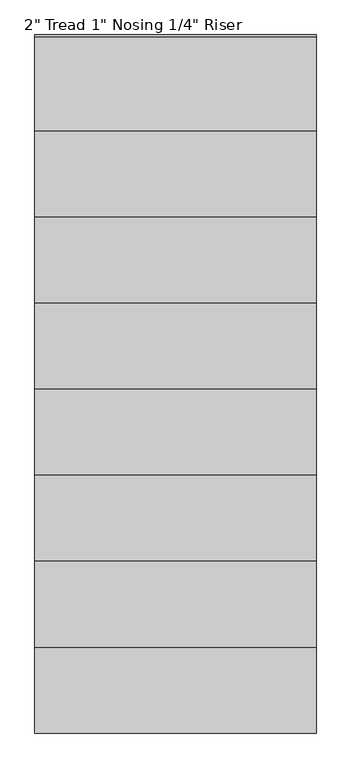
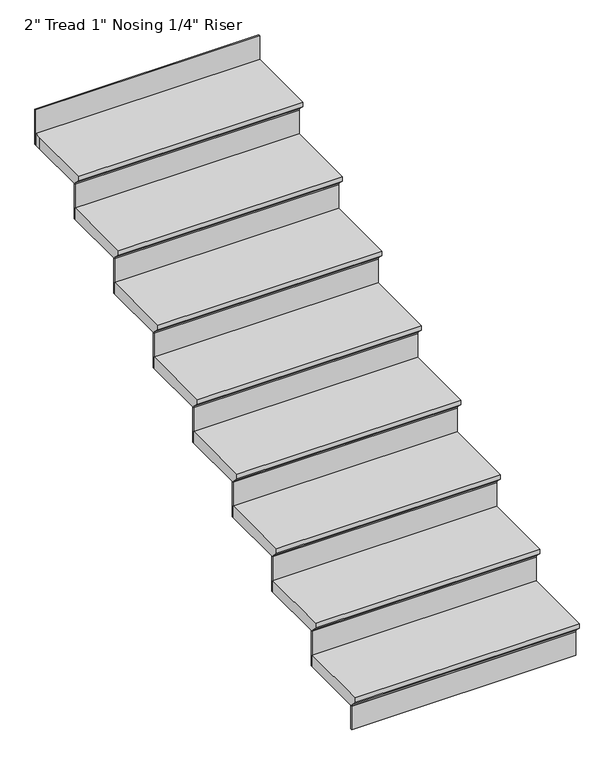
"""IFC4 building model written with IfcOpenShell, lengths in millimetres: stair flight geometry."""

from ifc_helpers import new_model, si_unit, origin, place, context, project, spatial, faceted_brep, source, transform, mapped, element, save


def stair_flight_7b1ec15d(model_context):
    return source(origin(), model_context, "Body", "Brep", [
        faceted_brep([(1196.7463194, 2224.4726898, 133.35), (1196.7463194, 2224.4726898, 152.4), (282.3463194, 2224.4726898, 152.4), (282.3463194, 2224.4726898, 133.35), (1196.7463194, 2249.8726898, 107.95), (282.3463194, 2249.8726898, 107.95), (1196.7463194, 2529.2726898, 152.4), (282.3463194, 2529.2726898, 152.4), (282.3463194, 2249.8726898, 101.6), (282.3463194, 2529.2726898, 101.6), (1196.7463194, 2529.2726898, 101.6), (1196.7463194, 2249.8726898, 101.6)], [[[0, 1, 2, 3]], [[4, 0, 3, 5]], [[2, 1, 6, 7]], [[8, 9, 10, 11]], [[2, 7, 9, 8, 5, 3]], [[8, 11, 4, 5]], [[6, 1, 0, 4, 11, 10]], [[7, 6, 10, 9]]]),
        faceted_brep([(1196.7463194, 2249.8726898, 101.6), (1196.7463194, 2249.8726898, 0.0), (1196.7463194, 2256.2226898, 0.0), (1196.7463194, 2256.2226898, 101.6), (282.3463194, 2249.8726898, 101.6), (282.3463194, 2256.2226898, 101.6), (282.3463194, 2256.2226898, 0.0), (282.3463194, 2249.8726898, 0.0)], [[[0, 1, 2, 3]], [[4, 5, 6, 7]], [[1, 0, 4, 7]], [[2, 1, 7, 6]], [[3, 2, 6, 5]], [[0, 3, 5, 4]]]),
        faceted_brep([(1196.7463194, 2529.2726898, 254.0), (1196.7463194, 2529.2726898, 101.6), (1196.7463194, 2535.6226898, 101.6), (1196.7463194, 2535.6226898, 254.0), (282.3463194, 2529.2726898, 254.0), (282.3463194, 2535.6226898, 254.0), (282.3463194, 2535.6226898, 101.6), (282.3463194, 2529.2726898, 101.6)], [[[0, 1, 2, 3]], [[4, 5, 6, 7]], [[1, 0, 4, 7]], [[2, 1, 7, 6]], [[3, 2, 6, 5]], [[0, 3, 5, 4]]]),
        faceted_brep([(282.3463194, 2503.8726898, 304.8), (1196.7463194, 2503.8726898, 304.8), (1196.7463194, 2808.6726898, 304.8), (282.3463194, 2808.6726898, 304.8), (282.3463194, 2529.2726898, 254.0), (282.3463194, 2808.6726898, 254.0), (1196.7463194, 2808.6726898, 254.0), (1196.7463194, 2529.2726898, 254.0), (282.3463194, 2529.2726898, 260.35), (282.3463194, 2503.8726898, 285.75), (1196.7463194, 2529.2726898, 260.35), (1196.7463194, 2503.8726898, 285.75)], [[[0, 1, 2, 3]], [[4, 5, 6, 7]], [[0, 3, 5, 4, 8, 9]], [[4, 7, 10, 8]], [[2, 1, 11, 10, 7, 6]], [[3, 2, 6, 5]], [[11, 1, 0, 9]], [[10, 11, 9, 8]]]),
        faceted_brep([(1196.7463194, 2808.6726898, 406.4), (1196.7463194, 2808.6726898, 254.0), (1196.7463194, 2815.0226898, 254.0), (1196.7463194, 2815.0226898, 406.4), (282.3463194, 2808.6726898, 406.4), (282.3463194, 2815.0226898, 406.4), (282.3463194, 2815.0226898, 254.0), (282.3463194, 2808.6726898, 254.0)], [[[0, 1, 2, 3]], [[4, 5, 6, 7]], [[1, 0, 4, 7]], [[2, 1, 7, 6]], [[3, 2, 6, 5]], [[0, 3, 5, 4]]]),
        faceted_brep([(282.3463194, 2783.2726898, 457.2), (1196.7463194, 2783.2726898, 457.2), (1196.7463194, 3088.0726898, 457.2), (282.3463194, 3088.0726898, 457.2), (282.3463194, 2808.6726898, 406.4), (282.3463194, 3088.0726898, 406.4), (1196.7463194, 3088.0726898, 406.4), (1196.7463194, 2808.6726898, 406.4), (282.3463194, 2808.6726898, 412.75), (282.3463194, 2783.2726898, 438.15), (1196.7463194, 2808.6726898, 412.75), (1196.7463194, 2783.2726898, 438.15)], [[[0, 1, 2, 3]], [[4, 5, 6, 7]], [[0, 3, 5, 4, 8, 9]], [[4, 7, 10, 8]], [[2, 1, 11, 10, 7, 6]], [[3, 2, 6, 5]], [[11, 1, 0, 9]], [[10, 11, 9, 8]]]),
        faceted_brep([(1196.7463194, 3088.0726898, 558.8), (1196.7463194, 3088.0726898, 406.4), (1196.7463194, 3094.4226898, 406.4), (1196.7463194, 3094.4226898, 558.8), (282.3463194, 3088.0726898, 558.8), (282.3463194, 3094.4226898, 558.8), (282.3463194, 3094.4226898, 406.4), (282.3463194, 3088.0726898, 406.4)], [[[0, 1, 2, 3]], [[4, 5, 6, 7]], [[1, 0, 4, 7]], [[2, 1, 7, 6]], [[3, 2, 6, 5]], [[0, 3, 5, 4]]]),
        faceted_brep([(282.3463194, 3062.6726898, 609.6), (1196.7463194, 3062.6726898, 609.6), (1196.7463194, 3367.4726898, 609.6), (282.3463194, 3367.4726898, 609.6), (282.3463194, 3088.0726898, 558.8), (282.3463194, 3367.4726898, 558.8), (1196.7463194, 3367.4726898, 558.8), (1196.7463194, 3088.0726898, 558.8), (282.3463194, 3088.0726898, 565.15), (282.3463194, 3062.6726898, 590.55), (1196.7463194, 3088.0726898, 565.15), (1196.7463194, 3062.6726898, 590.55)], [[[0, 1, 2, 3]], [[4, 5, 6, 7]], [[0, 3, 5, 4, 8, 9]], [[4, 7, 10, 8]], [[2, 1, 11, 10, 7, 6]], [[3, 2, 6, 5]], [[11, 1, 0, 9]], [[10, 11, 9, 8]]]),
        faceted_brep([(1196.7463194, 3367.4726898, 711.2), (1196.7463194, 3367.4726898, 558.8), (1196.7463194, 3373.8226898, 558.8), (1196.7463194, 3373.8226898, 711.2), (282.3463194, 3367.4726898, 711.2), (282.3463194, 3373.8226898, 711.2), (282.3463194, 3373.8226898, 558.8), (282.3463194, 3367.4726898, 558.8)], [[[0, 1, 2, 3]], [[4, 5, 6, 7]], [[1, 0, 4, 7]], [[2, 1, 7, 6]], [[3, 2, 6, 5]], [[0, 3, 5, 4]]]),
        faceted_brep([(282.3463194, 3342.0726898, 762.0), (1196.7463194, 3342.0726898, 762.0), (1196.7463194, 3646.8726898, 762.0), (282.3463194, 3646.8726898, 762.0), (282.3463194, 3367.4726898, 711.2), (282.3463194, 3646.8726898, 711.2), (1196.7463194, 3646.8726898, 711.2), (1196.7463194, 3367.4726898, 711.2), (282.3463194, 3367.4726898, 717.55), (282.3463194, 3342.0726898, 742.95), (1196.7463194, 3367.4726898, 717.55), (1196.7463194, 3342.0726898, 742.95)], [[[0, 1, 2, 3]], [[4, 5, 6, 7]], [[0, 3, 5, 4, 8, 9]], [[4, 7, 10, 8]], [[2, 1, 11, 10, 7, 6]], [[3, 2, 6, 5]], [[11, 1, 0, 9]], [[10, 11, 9, 8]]]),
        faceted_brep([(1196.7463194, 3646.8726898, 863.6), (1196.7463194, 3646.8726898, 711.2), (1196.7463194, 3653.2226898, 711.2), (1196.7463194, 3653.2226898, 863.6), (282.3463194, 3646.8726898, 863.6), (282.3463194, 3653.2226898, 863.6), (282.3463194, 3653.2226898, 711.2), (282.3463194, 3646.8726898, 711.2)], [[[0, 1, 2, 3]], [[4, 5, 6, 7]], [[1, 0, 4, 7]], [[2, 1, 7, 6]], [[3, 2, 6, 5]], [[0, 3, 5, 4]]]),
        faceted_brep([(282.3463194, 3621.4726898, 914.4), (1196.7463194, 3621.4726898, 914.4), (1196.7463194, 3926.2726898, 914.4), (282.3463194, 3926.2726898, 914.4), (282.3463194, 3646.8726898, 863.6), (282.3463194, 3926.2726898, 863.6), (1196.7463194, 3926.2726898, 863.6), (1196.7463194, 3646.8726898, 863.6), (282.3463194, 3646.8726898, 869.95), (282.3463194, 3621.4726898, 895.35), (1196.7463194, 3646.8726898, 869.95), (1196.7463194, 3621.4726898, 895.35)], [[[0, 1, 2, 3]], [[4, 5, 6, 7]], [[0, 3, 5, 4, 8, 9]], [[4, 7, 10, 8]], [[2, 1, 11, 10, 7, 6]], [[3, 2, 6, 5]], [[11, 1, 0, 9]], [[10, 11, 9, 8]]]),
        faceted_brep([(1196.7463194, 3926.2726898, 1016.0), (1196.7463194, 3926.2726898, 863.6), (1196.7463194, 3932.6226898, 863.6), (1196.7463194, 3932.6226898, 1016.0), (282.3463194, 3926.2726898, 1016.0), (282.3463194, 3932.6226898, 1016.0), (282.3463194, 3932.6226898, 863.6), (282.3463194, 3926.2726898, 863.6)], [[[0, 1, 2, 3]], [[4, 5, 6, 7]], [[1, 0, 4, 7]], [[2, 1, 7, 6]], [[3, 2, 6, 5]], [[0, 3, 5, 4]]]),
        faceted_brep([(282.3463194, 3900.8726898, 1066.8), (1196.7463194, 3900.8726898, 1066.8), (1196.7463194, 4205.6726898, 1066.8), (282.3463194, 4205.6726898, 1066.8), (282.3463194, 3926.2726898, 1016.0), (282.3463194, 4205.6726898, 1016.0), (1196.7463194, 4205.6726898, 1016.0), (1196.7463194, 3926.2726898, 1016.0), (282.3463194, 3926.2726898, 1022.35), (282.3463194, 3900.8726898, 1047.75), (1196.7463194, 3926.2726898, 1022.35), (1196.7463194, 3900.8726898, 1047.75)], [[[0, 1, 2, 3]], [[4, 5, 6, 7]], [[0, 3, 5, 4, 8, 9]], [[4, 7, 10, 8]], [[2, 1, 11, 10, 7, 6]], [[3, 2, 6, 5]], [[11, 1, 0, 9]], [[10, 11, 9, 8]]]),
        faceted_brep([(1196.7463194, 4485.0726898, 1320.8), (1196.7463194, 4485.0726898, 1168.4), (1196.7463194, 4491.4226898, 1168.4), (1196.7463194, 4491.4226898, 1320.8), (282.3463194, 4485.0726898, 1320.8), (282.3463194, 4491.4226898, 1320.8), (282.3463194, 4491.4226898, 1168.4), (282.3463194, 4485.0726898, 1168.4)], [[[0, 1, 2, 3]], [[4, 5, 6, 7]], [[1, 0, 4, 7]], [[2, 1, 7, 6]], [[3, 2, 6, 5]], [[0, 3, 5, 4]]]),
        faceted_brep([(1196.7463194, 4205.6726898, 1168.4), (1196.7463194, 4205.6726898, 1016.0), (1196.7463194, 4212.0226898, 1016.0), (1196.7463194, 4212.0226898, 1168.4), (282.3463194, 4205.6726898, 1168.4), (282.3463194, 4212.0226898, 1168.4), (282.3463194, 4212.0226898, 1016.0), (282.3463194, 4205.6726898, 1016.0)], [[[0, 1, 2, 3]], [[4, 5, 6, 7]], [[1, 0, 4, 7]], [[2, 1, 7, 6]], [[3, 2, 6, 5]], [[0, 3, 5, 4]]]),
        faceted_brep([(282.3463194, 4485.0726898, 1219.2), (282.3463194, 4459.6726898, 1219.2), (282.3463194, 4180.2726898, 1219.2), (1196.7463194, 4180.2726898, 1219.2), (1196.7463194, 4485.0726898, 1219.2), (282.3463194, 4459.6726898, 1168.4), (282.3463194, 4485.0726898, 1168.4), (1196.7463194, 4485.0726898, 1168.4), (1196.7463194, 4205.6726898, 1168.4), (282.3463194, 4205.6726898, 1168.4), (282.3463194, 4205.6726898, 1174.75), (282.3463194, 4180.2726898, 1200.15), (1196.7463194, 4205.6726898, 1174.75), (1196.7463194, 4180.2726898, 1200.15)], [[[0, 1, 2, 3, 4]], [[5, 6, 7, 8, 9]], [[1, 0, 6, 5]], [[2, 1, 5, 9, 10, 11]], [[9, 8, 12, 10]], [[4, 3, 13, 12, 8, 7]], [[0, 4, 7, 6]], [[13, 3, 2, 11]], [[12, 13, 11, 10]]]),
    ])


if __name__ == "__main__":
    model = new_model("IFC4")
    model_context = context("Model", 3, world=origin())
    ifc_project = project(units=[si_unit("LENGTHUNIT", "METRE", prefix="MILLI")], contexts=[model_context])
    site = spatial("IfcSite", under=ifc_project)
    building = spatial("IfcBuilding", under=site)
    placement = place(None, origin())
    stair_flight_shape = stair_flight_7b1ec15d(model_context)
    element("IfcStairFlight", 1, ObjectType="2\" Tread 1\" Nosing 1/4\" Riser", at=placement, inside=building, context=model_context, shape_type="MappedRepresentation", body=[
        mapped(stair_flight_shape, transform((0.0, 0.0, 0.0), x_axis=(1.0, 0.0, 0.0), y_axis=(0.0, 1.0, 0.0), z_axis=(0.0, 0.0, 1.0))),
    ])
    save(model, "model.ifc")
